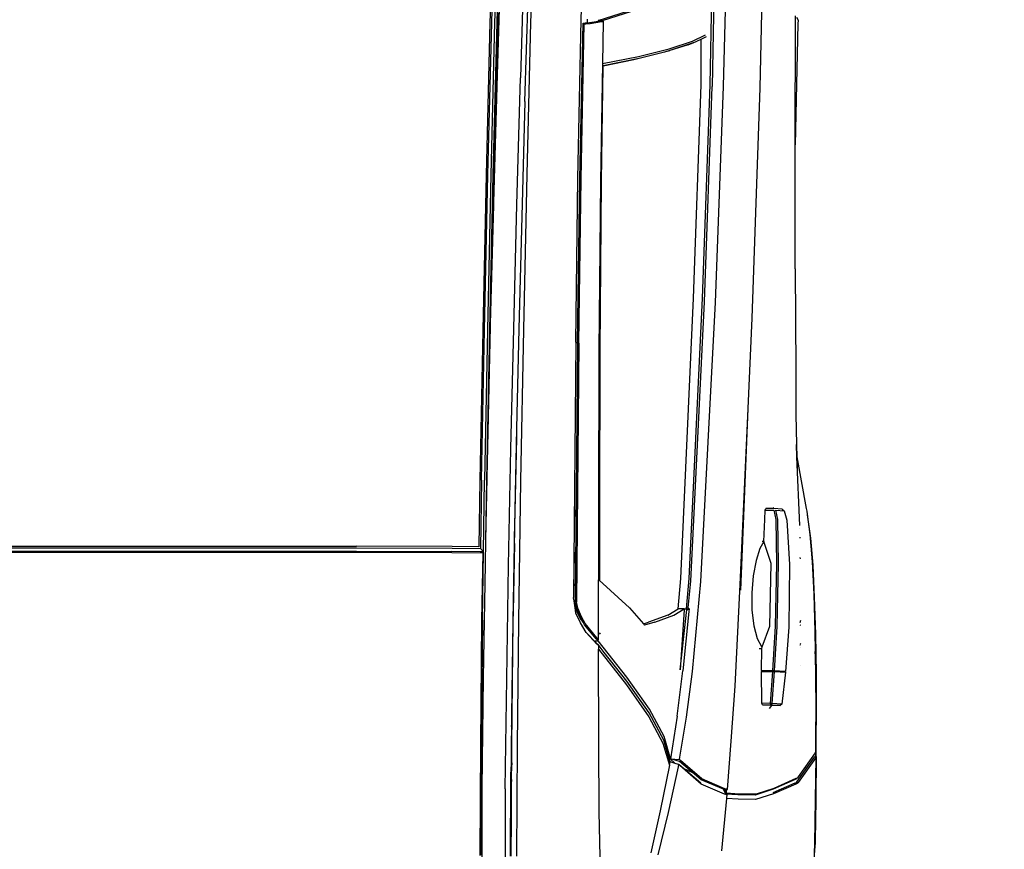
# Model space of a CAD drawing. Units: inches. Extents: x 1319 to 2030, y 219 to 1069.
# Tile 11 of 28: x 1461 to 1506, y 392 to 430. Entities that reach past the tile are written whole.
import ezdxf

# ---------------------------------------------------------------- set-up
doc = ezdxf.new("R2010")
doc.units = ezdxf.units.IN
doc.header["$MEASUREMENT"] = 0
doc.layers.get('0').update_dxf_attribs({"color": 12})
doc.layers.add('A-ANNO-DIMS', color=2, linetype='Continuous', lineweight=18)
doc.layers.add('C-PRKG-VEHC', color=8, linetype='Continuous', lineweight=13)
doc.layers.add('Edges', color=250, linetype='Continuous')
doc.styles.get("Standard").update_dxf_attribs({"font": 'arial.ttf'})
doc.dimstyles.get("Standard").update_dxf_attribs({"dimtxt": 7, "dimasz": 0.18, "dimexe": 0.18, "dimexo": 0.0625, "dimgap": 0.09, "dimtad": 0, "dimtih": 1, "dimtoh": 1, "dimzin": 0, "dimdsep": 46, "dimlunit": 3, "dimtxsty": 'Standard', "dimcen": 0.09, "dimadec": 0, "dimazin": 0, "dimtfac": 1, "dimtofl": 0, "dimtmove": 0, "dimatfit": 3, "dimfxl": 1, "dimtolj": 1, "dimtzin": 0, "dimarcsym": 0})

# ---------------------------------------------------------------- blocks, each defined once
blk = doc.blocks.new('Nissan Qashqai pl')
at = {"layer": 'Edges'}
for p, q in [((10.4339, 12.8061), (10.4573, 12.8093)), ((10.4345, 12.8062), (10.4613, 12.8099)), ((10.4573, 12.8093), (10.4889, 12.8119)), ((10.4613, 12.8099), (10.4926, 12.8125)), ((10.4889, 12.8119), (10.526, 12.8138)), ((10.4926, 12.8125), (10.5294, 12.8143)), ((10.526, 12.8138), (10.569, 12.8151)), ((10.5294, 12.8143), (10.5719, 12.8156)), ((10.569, 12.8151), (10.5919, 12.8155)), ((10.5719, 12.8156), (10.6176, 12.8164)), ((10.5919, 12.8155), (10.6151, 12.8159)), ((10.5981, 12.8157), (10.5919, 12.8155)), ((10.6174, 12.816), (10.5981, 12.8157)), ((10.6151, 12.8159), (10.6644, 12.8162)), ((10.6176, 12.8164), (10.6651, 12.8167)), ((10.6644, 12.8162), (10.7078, 12.8159)), ((10.6651, 12.8167), (10.666, 12.8167)), ((10.666, 12.8167), (10.677, 12.8167)), ((10.6729, 12.8157), (10.7082, 12.8156)), ((10.6809, 12.8167), (10.677, 12.8167)), ((10.7128, 12.8166), (10.6809, 12.8167)), ((10.7078, 12.8159), (10.7083, 12.8156)), ((10.7082, 12.8156), (10.7078, 12.8159)), ((10.7085, 12.8153), (10.7082, 12.8156)), ((10.7082, 12.8156), (10.7083, 12.8156)), ((10.7083, 12.8156), (10.7087, 12.8153)), ((10.7083, 12.8156), (10.7125, 12.8156)), ((10.7087, 12.8153), (10.7363, 12.7959)), ((10.7139, 12.8164), (10.7125, 12.8156)), ((10.7137, 12.8148), (10.7125, 12.8156)), ((10.7128, 12.8166), (10.7625, 12.8161)), ((10.7128, 12.8166), (10.724, 12.8166)), ((10.7137, 12.8148), (10.7138, 12.8147)), ((10.7418, 12.7947), (10.7138, 12.8147)), ((10.7139, 12.8164), (10.7148, 12.8157)), ((10.7628, 12.8158), (10.7139, 12.8164)), ((10.7148, 12.8157), (10.7429, 12.7956)), ((10.7685, 12.8161), (10.724, 12.8166)), ((10.7625, 12.8161), (10.7628, 12.8161)), ((10.7628, 12.8161), (10.8099, 12.8152)), ((10.8131, 12.8149), (10.7628, 12.8158)), ((10.7688, 12.8161), (10.7685, 12.8161)), ((10.8099, 12.8152), (10.7688, 12.8161)), ((10.8099, 12.8152), (10.8131, 12.8152)), ((10.8134, 12.8152), (10.8131, 12.8152)), ((10.8644, 12.8135), (10.8131, 12.8149)), ((10.8134, 12.8152), (10.8142, 12.8152)), ((10.8142, 12.8152), (10.8142, 12.8152)), ((10.8237, 12.8149), (10.8142, 12.8152)), ((10.3679, 12.7944), (10.4275, 12.8051)), ((10.4468, 12.7976), (10.3679, 12.7944)), ((10.4275, 12.8051), (10.4304, 12.8056)), ((10.4304, 12.8056), (10.4339, 12.8061)), ((10.4339, 12.8061), (10.4345, 12.8062)), ((10.4503, 12.7976), (10.4502, 12.7976)), ((10.4603, 12.7976), (10.4613, 12.7978)), ((10.4838, 12.7977), (10.4852, 12.7982)), ((10.5565, 12.7985), (10.5591, 12.7977)), ((10.5615, 12.7978), (10.5617, 12.7985)), ((10.583, 12.7984), (10.5834, 12.798)), ((10.5836, 12.798), (10.5831, 12.7984)), ((10.5847, 12.798), (10.5841, 12.7984)), ((10.5873, 12.7981), (10.5873, 12.7981)), ((10.6087, 12.7983), (10.6087, 12.7984)), ((9.8643, 12.7927), (9.8598, 12.7928)), ((9.8614, 12.7937), (9.8647, 12.7956)), ((10.0085, 12.7922), (9.8643, 12.7927)), ((9.8647, 12.7956), (9.869, 12.7954)), ((9.869, 12.7954), (10.0085, 12.7922)), ((10.0124, 12.7922), (10.0085, 12.7922)), ((10.1513, 12.7924), (10.0124, 12.7922)), ((10.1513, 12.7924), (10.2677, 12.793)), ((10.2677, 12.793), (10.3189, 12.7931)), ((10.3189, 12.7931), (10.3537, 12.7939)), ((10.3537, 12.7939), (10.3832, 12.7945)), ((10.3679, 12.7944), (10.3537, 12.7939)), ((10.4406, 12.7829), (10.4919, 12.7858)), ((10.4919, 12.7858), (10.564, 12.7851)), ((10.7363, 12.7959), (10.7376, 12.795)), ((10.7387, 12.794), (10.7376, 12.795)), ((10.7376, 12.795), (10.7378, 12.7946)), ((10.7378, 12.7946), (10.7379, 12.7945)), ((10.7378, 12.7946), (10.7385, 12.7932)), ((10.7385, 12.7932), (10.7497, 12.7679)), ((10.7387, 12.794), (10.7396, 12.7922)), ((10.7396, 12.7922), (10.7507, 12.7669)), ((10.743, 12.7939), (10.7418, 12.7947)), ((10.7432, 12.7954), (10.7426, 12.7954)), ((10.7429, 12.7956), (10.7432, 12.7954)), ((10.7434, 12.793), (10.743, 12.7939)), ((10.7441, 12.7954), (10.7432, 12.7954)), ((10.7432, 12.7954), (10.744, 12.7948)), ((10.7437, 12.7921), (10.7434, 12.793)), ((10.7438, 12.7921), (10.7437, 12.7921)), ((10.7438, 12.7921), (10.7549, 12.7666)), ((10.744, 12.7948), (10.7448, 12.793)), ((10.7448, 12.793), (10.7559, 12.7674)), ((10.4282, 12.7775), (10.4274, 12.7679)), ((10.4282, 12.7775), (10.4299, 12.7798)), ((10.4291, 12.77), (10.4299, 12.7798)), ((10.4299, 12.7798), (10.4406, 12.7829)), ((10.564, 12.7851), (10.6151, 12.7813)), ((10.615, 12.7803), (10.6142, 12.7686)), ((10.6151, 12.7813), (10.615, 12.7803)), ((10.615, 12.7676), (10.6151, 12.7803)), ((10.6151, 12.7803), (10.615, 12.7803)), ((10.6151, 12.7803), (10.6151, 12.7813)), ((10.6151, 12.7685), (10.616, 12.7812)), ((10.616, 12.7812), (10.6526, 12.7768)), ((10.6526, 12.7768), (10.6518, 12.7657)), ((10.6526, 12.7768), (10.6543, 12.7749)), ((10.6537, 12.7658), (10.6543, 12.7749)), ((10.6543, 12.7749), (10.6543, 12.7656)), ((10.4263, 12.7665), (10.4274, 12.7674)), ((10.4274, 12.7679), (10.4274, 12.7674)), ((10.4274, 12.7674), (10.4275, 12.7586)), ((10.4398, 12.7724), (10.4291, 12.77)), ((10.4291, 12.7677), (10.4398, 12.7701)), ((10.4293, 12.7579), (10.4291, 12.7677)), ((10.4909, 12.773), (10.4398, 12.7724)), ((10.4398, 12.7701), (10.4909, 12.7708)), ((10.4908, 12.7648), (10.4653, 12.7564)), ((10.563, 12.7633), (10.4908, 12.7648)), ((10.5631, 12.7715), (10.4909, 12.773)), ((10.4909, 12.7708), (10.563, 12.7692)), ((10.563, 12.7692), (10.6142, 12.7663)), ((10.5867, 12.7545), (10.563, 12.7633)), ((10.6142, 12.7686), (10.5631, 12.7715)), ((10.6142, 12.766), (10.6141, 12.7537)), ((10.6142, 12.7686), (10.6142, 12.7677)), ((10.6142, 12.7677), (10.615, 12.7676)), ((10.6142, 12.7677), (10.6142, 12.7663)), ((10.6142, 12.7663), (10.6142, 12.766)), ((10.6151, 12.7676), (10.615, 12.7676)), ((10.615, 12.7537), (10.6151, 12.7659)), ((10.6518, 12.7657), (10.6151, 12.7685)), ((10.6151, 12.7676), (10.6151, 12.7685)), ((10.6151, 12.7662), (10.6151, 12.7676)), ((10.6151, 12.7662), (10.6518, 12.7634)), ((10.6151, 12.7659), (10.6151, 12.7662)), ((10.6518, 12.7634), (10.6517, 12.754)), ((10.6536, 12.7639), (10.6518, 12.7657)), ((10.6518, 12.7657), (10.6518, 12.7634)), ((10.6518, 12.7634), (10.6536, 12.7639)), ((10.6543, 12.7656), (10.6535, 12.7546)), ((10.6535, 12.7546), (10.6536, 12.7639)), ((10.6536, 12.7639), (10.6537, 12.7658)), ((10.6537, 12.7658), (10.6543, 12.7656)), ((10.6578, 12.7628), (10.6543, 12.7656)), ((10.7497, 12.7679), (10.7565, 12.7473)), ((10.7507, 12.7669), (10.7575, 12.7462)), ((10.7559, 12.7674), (10.7626, 12.7467)), ((9.8024, 12.7549), (9.9426, 12.7518)), ((9.9426, 12.7518), (10.2081, 12.7424)), ((10.4293, 12.7579), (10.4275, 12.7586)), ((10.4398, 12.7573), (10.4293, 12.7579)), ((10.4653, 12.7564), (10.4398, 12.7573)), ((10.4653, 12.7561), (10.4652, 12.7545)), ((10.4653, 12.7564), (10.4653, 12.7561)), ((10.4653, 12.7564), (10.4653, 12.7564)), ((10.4653, 12.7564), (10.4653, 12.7561)), ((10.4653, 12.7561), (10.4653, 12.7561)), ((10.4653, 12.7561), (10.4732, 12.7517)), ((10.4732, 12.7517), (10.4871, 12.7474)), ((10.5769, 12.7484), (10.5863, 12.7537)), ((10.5863, 12.7537), (10.5867, 12.7545)), ((10.5885, 12.7538), (10.5867, 12.7545)), ((10.5885, 12.751), (10.5885, 12.7538)), ((10.6141, 12.7537), (10.5885, 12.7538)), ((10.6141, 12.7537), (10.615, 12.7537)), ((10.6517, 12.754), (10.615, 12.7537)), ((10.6535, 12.7546), (10.6517, 12.754)), ((10.2081, 12.7424), (10.312, 12.7377)), ((10.4871, 12.7474), (10.5048, 12.744)), ((10.5048, 12.744), (10.5246, 12.7423)), ((10.5246, 12.7423), (10.5445, 12.7425)), ((10.5445, 12.7425), (10.5625, 12.7446)), ((10.5625, 12.7446), (10.5769, 12.7484)), ((10.7565, 12.7473), (10.7563, 12.7273)), ((10.7575, 12.7462), (10.7572, 12.7263)), ((10.7626, 12.7467), (10.7623, 12.7269)), ((10.312, 12.7377), (10.5214, 12.7293)), ((10.312, 12.7377), (10.5147, 12.7285)), ((10.5147, 12.7285), (10.6318, 12.7228)), ((10.6318, 12.7228), (10.6955, 12.7184)), ((10.6955, 12.7184), (10.7509, 12.714)), ((10.7563, 12.7273), (10.7553, 12.7134)), ((10.7572, 12.7263), (10.7563, 12.7126)), ((10.7623, 12.7269), (10.7615, 12.7131)), ((9.9414, 12.71), (9.8143, 12.713)), ((10.19, 12.7008), (9.9414, 12.71)), ((10.7501, 12.7114), (10.7387, 12.6849)), ((10.7507, 12.7098), (10.7397, 12.684)), ((10.7563, 12.7109), (10.7449, 12.6843)), ((10.7507, 12.7132), (10.7501, 12.7114)), ((10.7506, 12.7111), (10.7507, 12.7132)), ((10.7507, 12.7132), (10.7509, 12.714)), ((10.751, 12.7132), (10.7507, 12.7132)), ((10.7511, 12.7107), (10.7507, 12.7098)), ((10.7524, 12.7106), (10.7507, 12.7098)), ((10.7522, 12.7131), (10.7509, 12.714)), ((10.7516, 12.7131), (10.7509, 12.714)), ((10.7519, 12.7128), (10.7511, 12.7107)), ((10.7522, 12.7131), (10.7516, 12.7131)), ((10.7519, 12.7128), (10.7516, 12.7131)), ((10.7526, 12.7124), (10.7519, 12.7128)), ((10.7553, 12.7134), (10.7522, 12.7131)), ((10.7524, 12.7106), (10.7526, 12.7124)), ((10.7556, 12.7122), (10.7524, 12.7106)), ((10.7526, 12.7124), (10.7526, 12.7127)), ((10.7532, 12.712), (10.7526, 12.7124)), ((10.7556, 12.7122), (10.7532, 12.712)), ((10.7561, 12.7125), (10.7556, 12.7122)), ((10.7561, 12.7125), (10.7563, 12.7126)), ((10.7563, 12.7125), (10.7561, 12.7125)), ((10.7563, 12.7123), (10.7561, 12.7123)), ((10.7563, 12.7126), (10.7573, 12.7135)), ((10.7563, 12.7126), (10.7563, 12.7125)), ((10.7569, 12.7125), (10.7563, 12.7109)), ((10.7569, 12.7125), (10.7563, 12.7125)), ((10.7563, 12.7125), (10.7563, 12.7123)), ((10.7573, 12.7135), (10.7569, 12.7125)), ((10.7573, 12.7135), (10.7604, 12.7132)), ((10.7604, 12.7132), (10.7615, 12.7131)), ((10.7615, 12.7131), (10.8218, 12.7077)), ((9.8101, 12.6993), (9.9411, 12.6966)), ((9.9393, 12.6944), (9.8119, 12.697)), ((10.1894, 12.6879), (9.9411, 12.6966)), ((10.5113, 12.6839), (10.19, 12.7008)), ((9.8891, 12.6741), (9.8818, 12.6891)), ((9.8867, 12.6842), (9.8838, 12.6901)), ((9.9393, 12.684), (9.8867, 12.6842)), ((9.8911, 12.675), (9.8867, 12.6842)), ((10.1849, 12.6857), (9.9393, 12.6944)), ((10.1849, 12.6754), (9.9393, 12.684)), ((10.5079, 12.6703), (10.1849, 12.6857)), ((10.5109, 12.6721), (10.1894, 12.6879)), ((10.6152, 12.674), (10.5113, 12.6839)), ((10.7387, 12.6849), (10.7177, 12.6604)), ((10.7449, 12.6843), (10.7232, 12.6594)), ((10.7438, 12.6836), (10.7265, 12.6635)), ((10.7397, 12.684), (10.7334, 12.6766)), ((9.8978, 12.6472), (9.8891, 12.6741)), ((9.8911, 12.6749), (9.8911, 12.675)), ((9.8931, 12.6691), (9.8911, 12.6749)), ((9.8911, 12.6749), (9.8998, 12.6481)), ((10.5079, 12.6607), (10.1849, 12.6754)), ((10.6678, 12.6672), (10.6152, 12.674)), ((10.7334, 12.6766), (10.7186, 12.6593)), ((10.7265, 12.6635), (10.7316, 12.6741)), ((9.8931, 12.669), (9.8931, 12.6691)), ((9.8931, 12.669), (9.9018, 12.6421)), ((10.543, 12.6671), (10.5079, 12.6703)), ((10.5417, 12.6693), (10.5109, 12.6721)), ((10.5417, 12.6693), (10.5427, 12.6702)), ((10.5417, 12.6693), (10.543, 12.6671)), ((10.5436, 12.6687), (10.5427, 12.6702)), ((10.5427, 12.6702), (10.5458, 12.67)), ((10.544, 12.6678), (10.543, 12.6671)), ((10.543, 12.6646), (10.543, 12.6671)), ((10.543, 12.6646), (10.543, 12.6576)), ((10.5439, 12.6646), (10.543, 12.6646)), ((10.5502, 12.6526), (10.543, 12.6646)), ((10.544, 12.6678), (10.5436, 12.6687)), ((10.5439, 12.6646), (10.613, 12.6601)), ((10.547, 12.6674), (10.544, 12.6678)), ((10.5458, 12.67), (10.6144, 12.6629)), ((10.613, 12.6601), (10.547, 12.6674)), ((10.6664, 12.6566), (10.6144, 12.6629)), ((10.7137, 12.6595), (10.6678, 12.6672)), ((10.7265, 12.6635), (10.7224, 12.6587)), ((10.543, 12.6576), (10.5079, 12.6607)), ((10.5502, 12.6456), (10.543, 12.6576)), ((10.5584, 12.6306), (10.5502, 12.6526)), ((10.6664, 12.6566), (10.7155, 12.649)), ((10.7165, 12.6591), (10.7137, 12.6595)), ((10.7186, 12.6593), (10.7155, 12.649)), ((10.7155, 12.649), (10.7165, 12.6591)), ((10.7209, 12.654), (10.7155, 12.6485)), ((10.7177, 12.6604), (10.7165, 12.6591)), ((10.7209, 12.654), (10.7192, 12.6484)), ((10.7221, 12.6581), (10.7209, 12.654)), ((10.7232, 12.6594), (10.7221, 12.6581)), ((10.7221, 12.6581), (10.7224, 12.6587)), ((10.7221, 12.6581), (10.7247, 12.6575)), ((10.7247, 12.6575), (10.7776, 12.646)), ((9.9066, 12.6119), (9.8978, 12.6472)), ((9.9086, 12.6129), (9.8998, 12.6481)), ((9.9018, 12.6421), (9.9106, 12.6068)), ((10.5502, 12.6456), (10.5584, 12.6236)), ((10.69, 12.6414), (10.6583, 12.6245)), ((10.6943, 12.641), (10.6627, 12.6241)), ((10.6671, 12.6238), (10.6976, 12.6401)), ((10.7155, 12.649), (10.69, 12.6414)), ((10.7155, 12.6473), (10.6943, 12.641)), ((10.6976, 12.6401), (10.7228, 12.6477)), ((10.7155, 12.649), (10.7155, 12.6485)), ((10.7155, 12.6485), (10.7155, 12.6473)), ((10.7192, 12.6484), (10.7155, 12.6473)), ((10.7228, 12.6477), (10.7192, 12.6484)), ((10.7228, 12.6477), (10.7754, 12.637)), ((10.7776, 12.646), (10.8264, 12.6341)), ((10.5584, 12.6306), (10.5617, 12.619)), ((10.7754, 12.637), (10.8239, 12.6261)), ((10.5419, 12.6018), (10.56, 12.6176)), ((10.56, 12.6176), (10.5584, 12.6236)), ((10.56, 12.6176), (10.5617, 12.619)), ((10.6583, 12.6245), (10.6215, 12.5986)), ((10.6627, 12.6241), (10.6261, 12.5984)), ((10.6306, 12.5982), (10.6671, 12.6238)), ((9.8652, 12.5704), (9.8516, 12.6129)), ((9.8652, 12.5654), (9.8516, 12.6079)), ((9.9149, 12.5705), (9.9066, 12.6119)), ((9.9169, 12.5714), (9.9086, 12.6129)), ((9.9106, 12.6068), (9.9177, 12.5714)), ((10.51, 12.5666), (10.5419, 12.6018)), ((10.6215, 12.5986), (10.5796, 12.5655)), ((10.5892, 12.5659), (10.6306, 12.5982)), ((10.6261, 12.5984), (10.593, 12.5726)), ((9.8652, 12.5706), (9.8664, 12.5714)), ((9.8652, 12.5706), (9.8665, 12.5695)), ((9.8652, 12.5704), (9.8652, 12.5706)), ((9.8652, 12.5704), (9.8652, 12.5704)), ((9.8652, 12.5704), (9.8652, 12.5654)), ((9.8655, 12.5687), (9.8652, 12.5704)), ((9.8665, 12.5695), (9.8664, 12.5714)), ((9.8664, 12.5714), (9.9149, 12.5705)), ((9.9149, 12.5705), (10.0505, 12.5681)), ((9.9177, 12.5714), (9.9169, 12.5714)), ((10.0501, 12.5695), (9.9177, 12.5714)), ((10.593, 12.5726), (10.584, 12.5655)), ((9.8675, 12.5555), (9.8655, 12.5687)), ((9.8686, 12.5562), (9.8665, 12.5695)), ((10.2453, 12.568), (10.0501, 12.5695)), ((10.0505, 12.5681), (10.2453, 12.5664)), ((10.4292, 12.5674), (10.2453, 12.568)), ((10.2453, 12.5664), (10.4289, 12.5658)), ((10.4289, 12.5658), (10.5092, 12.5658)), ((10.5099, 12.5674), (10.4292, 12.5674)), ((10.5099, 12.5674), (10.5092, 12.5658)), ((10.5092, 12.5658), (10.5094, 12.5658)), ((10.5094, 12.5658), (10.51, 12.5666)), ((10.5783, 12.5659), (10.5094, 12.5658)), ((10.51, 12.5666), (10.5099, 12.5674)), ((10.5764, 12.5642), (10.5598, 12.5507)), ((10.5776, 12.5633), (10.5612, 12.5498)), ((10.5834, 12.5641), (10.57, 12.5517)), ((10.57, 12.5517), (10.5821, 12.5633)), ((10.5709, 12.5675), (10.5705, 12.5671)), ((10.5719, 12.5682), (10.5709, 12.5675)), ((10.5783, 12.5659), (10.5764, 12.5642)), ((10.5776, 12.5633), (10.5783, 12.5659)), ((10.5796, 12.5655), (10.5776, 12.5633)), ((10.5796, 12.5655), (10.5783, 12.5659)), ((10.5796, 12.562), (10.5796, 12.5655)), ((10.5838, 12.5653), (10.5821, 12.5633)), ((10.584, 12.5647), (10.5834, 12.5641)), ((10.584, 12.5655), (10.5838, 12.5653)), ((10.584, 12.5655), (10.5841, 12.5655)), ((10.584, 12.5654), (10.584, 12.5655)), ((10.5847, 12.5655), (10.584, 12.5647)), ((10.584, 12.5647), (10.584, 12.5654)), ((10.5851, 12.5659), (10.5841, 12.5655)), ((10.5841, 12.5655), (10.5847, 12.5655)), ((10.5851, 12.5659), (10.5847, 12.5655)), ((10.5851, 12.5659), (10.5892, 12.5659)), ((10.6988, 12.5662), (10.5892, 12.5659)), ((10.7769, 12.5667), (10.6988, 12.5662)), ((10.858, 12.5683), (10.7769, 12.5667)), ((9.8644, 12.5459), (9.696, 12.551)), ((9.8643, 12.5532), (9.8637, 12.5532)), ((9.8677, 12.5531), (9.8643, 12.5532)), ((9.8677, 12.5531), (9.8675, 12.5555)), ((9.8678, 12.5507), (9.8677, 12.5531)), ((9.8681, 12.5482), (9.8678, 12.5507)), ((9.8681, 12.5482), (9.869, 12.5496)), ((10.0476, 12.5445), (9.8681, 12.5482)), ((9.8689, 12.5515), (9.8686, 12.5562)), ((9.869, 12.5496), (9.8689, 12.5515)), ((10.0477, 12.5459), (9.869, 12.5496)), ((10.5598, 12.5507), (10.5522, 12.5465)), ((10.5583, 12.5481), (10.5546, 12.546)), ((10.5551, 12.5457), (10.5583, 12.5481)), ((10.5612, 12.5498), (10.5583, 12.5481)), ((10.57, 12.5517), (10.5589, 12.5451)), ((10.0472, 12.5423), (9.8644, 12.5459)), ((10.2357, 12.5398), (10.0472, 12.5423)), ((10.2367, 12.5419), (10.0476, 12.5445)), ((10.2369, 12.5433), (10.0477, 12.5459)), ((10.2357, 12.5398), (10.53, 12.5373)), ((10.2367, 12.5419), (10.5351, 12.5392)), ((10.2369, 12.5433), (10.5348, 12.5406)), ((10.4153, 12.5384), (10.4176, 12.5384)), ((10.4176, 12.5384), (10.4181, 12.5384)), ((10.4181, 12.5384), (10.4552, 12.538)), ((10.4181, 12.5384), (10.4181, 12.5384)), ((10.4778, 12.5378), (10.53, 12.5373)), ((10.5301, 12.5373), (10.53, 12.5373)), ((10.5335, 12.5378), (10.5301, 12.5373)), ((10.5419, 12.5391), (10.5335, 12.5378)), ((10.5422, 12.542), (10.5348, 12.5406)), ((10.5418, 12.5405), (10.5351, 12.5392)), ((10.5424, 12.5406), (10.5418, 12.5405)), ((10.5419, 12.5391), (10.5463, 12.541)), ((10.5479, 12.54), (10.5419, 12.5391)), ((10.5522, 12.5465), (10.5422, 12.542)), ((10.5495, 12.5438), (10.5424, 12.5406)), ((10.5463, 12.541), (10.5551, 12.5457)), ((10.5589, 12.5451), (10.5479, 12.54)), ((10.5546, 12.546), (10.5495, 12.5438)), ((9.7029, 12.4926), (9.8673, 12.4878)), ((9.9583, 12.4812), (9.651, 12.4906)), ((9.6514, 12.4849), (9.9312, 12.4761)), ((9.8673, 12.4878), (10.0423, 12.4835)), ((9.9583, 12.4812), (10.091, 12.4775)), ((10.0423, 12.4835), (10.2211, 12.4795)), ((10.0776, 12.4719), (9.9312, 12.4761)), ((10.2201, 12.4683), (10.0776, 12.4719)), ((10.091, 12.4775), (10.2202, 12.4743)), ((10.3586, 12.4651), (10.2201, 12.4683)), ((10.2202, 12.4743), (10.2203, 12.4743)), ((10.2203, 12.4743), (10.3353, 12.4717)), ((10.2211, 12.4795), (10.3955, 12.4762)), ((10.3353, 12.4717), (10.4477, 12.4694)), ((10.3353, 12.4717), (10.346, 12.4714)), ((10.346, 12.4714), (10.4477, 12.4694)), ((10.3955, 12.4762), (10.5572, 12.4737)), ((10.4477, 12.4694), (10.4538, 12.4693)), ((10.4538, 12.4693), (10.4681, 12.469)), ((10.4676, 12.4691), (10.4538, 12.4693)), ((10.5566, 12.4677), (10.4676, 12.4691)), ((10.4676, 12.4691), (10.546, 12.4677)), ((10.4681, 12.469), (10.5866, 12.467)), ((10.5572, 12.4737), (10.7004, 12.4722)), ((10.7004, 12.4722), (10.8279, 12.4715)), ((9.6472, 12.4581), (9.9278, 12.4492)), ((10.4931, 12.4624), (10.3586, 12.4651)), ((10.6237, 12.4603), (10.4931, 12.4624)), ((10.546, 12.4677), (10.546, 12.4678)), ((10.546, 12.4677), (10.5576, 12.4675)), ((10.7, 12.4662), (10.5566, 12.4677)), ((10.5576, 12.4675), (10.6649, 12.4659)), ((10.5866, 12.467), (10.6649, 12.4659)), ((10.7502, 12.4586), (10.6237, 12.4603)), ((10.6649, 12.4659), (10.6786, 12.4658)), ((10.6649, 12.4659), (10.6772, 12.4657)), ((10.6786, 12.4657), (10.6772, 12.4657)), ((10.6786, 12.4658), (10.6786, 12.4662)), ((10.6786, 12.4657), (10.6786, 12.4658)), ((10.6786, 12.4658), (10.6801, 12.4657)), ((10.6786, 12.4657), (10.6801, 12.4657)), ((10.6801, 12.4662), (10.6801, 12.4657)), ((10.6801, 12.4657), (10.6801, 12.4657)), ((10.6801, 12.4657), (10.6811, 12.4657)), ((10.6801, 12.4657), (10.6811, 12.4657)), ((10.6811, 12.4662), (10.6811, 12.4657)), ((10.6811, 12.4657), (10.6811, 12.4657)), ((10.6811, 12.4657), (10.6966, 12.4654)), ((10.6811, 12.4657), (10.6991, 12.4655)), ((10.6811, 12.4657), (10.6991, 12.4655)), ((10.6966, 12.4654), (10.7144, 12.4653)), ((10.6991, 12.4655), (10.7144, 12.4653)), ((10.7201, 12.4661), (10.7, 12.4662)), ((10.7144, 12.4653), (10.7239, 12.4653)), ((10.7201, 12.4661), (10.7306, 12.4653)), ((10.7395, 12.4659), (10.7201, 12.4661)), ((10.7239, 12.4653), (10.7248, 12.4653)), ((10.7306, 12.4653), (10.7248, 12.4653)), ((10.7311, 12.4652), (10.7306, 12.4653)), ((10.7495, 12.4652), (10.7311, 12.4652)), ((10.7311, 12.4652), (10.7502, 12.4651)), ((10.7395, 12.4659), (10.7495, 12.4652)), ((10.7923, 12.4656), (10.7395, 12.4659)), ((10.8179, 12.4648), (10.7495, 12.4652)), ((10.7502, 12.4651), (10.7504, 12.4651)), ((10.7502, 12.4586), (10.968, 12.4585)), ((10.7504, 12.4651), (10.7808, 12.4649)), ((10.7808, 12.4649), (10.8179, 12.4648)), ((10.7923, 12.4652), (10.7923, 12.4656)), ((10.7933, 12.4656), (10.7923, 12.4656)), ((10.7933, 12.4652), (10.7933, 12.4656)), ((10.804, 12.4656), (10.7933, 12.4656)), ((10.804, 12.4653), (10.804, 12.4656)), ((10.8075, 12.4655), (10.804, 12.4656)), ((10.8075, 12.4655), (10.8075, 12.4653)), ((10.811, 12.4655), (10.8075, 12.4655)), ((10.811, 12.4655), (10.811, 12.4653)), ((10.8145, 12.4655), (10.811, 12.4655)), ((10.8145, 12.4653), (10.8145, 12.4655)), ((10.8279, 12.4654), (10.8145, 12.4655)), ((10.8277, 12.4647), (10.8179, 12.4648)), ((9.701, 12.4459), (9.8673, 12.441)), ((9.8673, 12.443), (9.7011, 12.4478)), ((9.7014, 12.4536), (9.8673, 12.4488)), ((9.7014, 12.4513), (9.8673, 12.4464)), ((9.9794, 12.4475), (9.8565, 12.451)), ((9.8673, 12.4488), (10.0429, 12.4444)), ((9.8673, 12.4464), (10.0429, 12.4421)), ((9.9278, 12.4492), (10.0747, 12.445)), ((10.0998, 12.4443), (9.9794, 12.4475)), ((10.043, 12.4387), (9.8673, 12.443)), ((9.8673, 12.441), (10.0431, 12.4367)), ((10.0429, 12.4444), (10.2216, 12.4404)), ((10.0429, 12.4421), (10.2215, 12.4381)), ((10.2218, 12.4347), (10.043, 12.4387)), ((10.0431, 12.4367), (10.2218, 12.4327)), ((10.0747, 12.445), (10.078, 12.4449)), ((10.078, 12.4449), (10.2146, 12.4414)), ((10.2146, 12.4414), (10.0998, 12.4443)), ((10.2146, 12.4414), (10.2175, 12.4413)), ((10.2175, 12.4413), (10.3564, 12.4382)), ((10.2215, 12.4381), (10.3945, 12.4348)), ((10.2216, 12.4404), (10.3947, 12.4371)), ((10.3947, 12.4314), (10.2218, 12.4347)), ((10.3564, 12.4382), (10.4638, 12.436)), ((10.4773, 12.4335), (10.3945, 12.4348)), ((10.3947, 12.4371), (10.4638, 12.436)), ((10.4638, 12.436), (10.4914, 12.4355)), ((10.4914, 12.4355), (10.6223, 12.4333)), ((10.2218, 12.4327), (10.3947, 12.4294)), ((10.3947, 12.4314), (10.4735, 12.4301)), ((10.3947, 12.4294), (10.4715, 12.4282)), ((10.4715, 12.4282), (10.4711, 12.3973)), ((10.4731, 12.3973), (10.4735, 12.4301)), ((10.4735, 12.4301), (10.4773, 12.4335)), ((10.4773, 12.4296), (10.4769, 12.3968)), ((10.4773, 12.4335), (10.4773, 12.4296)), ((10.4785, 12.433), (10.4773, 12.4335)), ((10.5561, 12.4323), (10.4773, 12.4335)), ((10.4781, 12.3972), (10.4785, 12.433)), ((10.5563, 12.4318), (10.4785, 12.433)), ((10.5561, 12.4323), (10.6996, 12.4308)), ((10.6999, 12.4304), (10.5563, 12.4318)), ((10.6223, 12.4333), (10.7493, 12.4316)), ((10.6996, 12.4308), (10.7722, 12.4304)), ((10.827, 12.4297), (10.6999, 12.4304)), ((10.7493, 12.4316), (11.0294, 12.4315)), ((10.7722, 12.4304), (10.7722, 12.4302)), ((10.7722, 12.4304), (10.7889, 12.4303)), ((10.7889, 12.4302), (10.7889, 12.4303)), ((10.7889, 12.4303), (10.7923, 12.4303)), ((10.7923, 12.4302), (10.7923, 12.4303)), ((10.7923, 12.4303), (10.7933, 12.4303)), ((10.7933, 12.4302), (10.7933, 12.4303)), ((10.7933, 12.4303), (10.8267, 12.4301)), ((10.4711, 12.3973), (10.4706, 12.2875)), ((10.4726, 12.2875), (10.4731, 12.3973)), ((10.4764, 12.2872), (10.4769, 12.3968)), ((10.4776, 12.2874), (10.4781, 12.3972)), ((10.4706, 11.5566), (10.4706, 12.2875)), ((10.4726, 11.5567), (10.4726, 12.2875)), ((10.4764, 11.5569), (10.4764, 12.2872)), ((10.4776, 11.5567), (10.4776, 12.2874))]:
    blk.add_line(p, q, dxfattribs=at)
blk = doc.blocks.new('car')
blk.add_blockref('Nissan Qashqai pl', (-9.7433, -11.9151))
blk = doc.blocks.new('carr')
blk.add_blockref('car', (0.5124, -0.007))
blk = doc.blocks.new('*D65')
at = {"layer": 'A-ANNO-DIMS', "color": 0, "lineweight": -2, "transparency": 16777216}
for p, q in [((1648.280254, 472.227245), (1329.112754, 472.227245)), ((1329.292754, 472.047245), (1329.292754, 431.817245)), ((1329.292754, 384.407245), (1329.292754, 424.637245)), ((1648.280254, 384.227245), (1329.112754, 384.227245))]:
    blk.add_line(p, q, dxfattribs=at)
at = {"layer": 'A-ANNO-DIMS', "color": 0, "transparency": 16777216}
for points in [[(1329.262754, 472.047245), (1329.322754, 472.047245), (1329.292754, 472.227245)], [(1329.262754, 384.407245), (1329.322754, 384.407245), (1329.292754, 384.227245)]]:
    blk.add_solid(points, dxfattribs=at)
at = {"layer": 'Defpoints', "color": 0, "transparency": 16777216}
for p in [(1329.292754, 472.227245), (1648.342754, 472.227245), (1648.342754, 384.227245)]:
    blk.add_point(p, dxfattribs=at)
at = {"layer": 'A-ANNO-DIMS', "color": 0, "transparency": 16777216, "insert": (1329.292754, 428.227245), "char_height": 7, "attachment_point": 5}
blk.add_mtext('\\A1;7\'-4"', dxfattribs=at)

msp = doc.modelspace()

# ---------------------------------------------------------------- block references
at = {"layer": 'C-PRKG-VEHC', "xscale": 39.37007874015748, "yscale": 39.37007874015748, "zscale": 39.37007874015748, "rotation": 270}
msp.add_blockref('carr', (1462.179, 454.621), dxfattribs=at)

# ---------------------------------------------------------------- dimensions: what is measured, and where the dimension line sits
at = {"layer": 'A-ANNO-DIMS'}
dim = msp.add_linear_dim(base=(1329.293, 472.227), p1=(1648.343, 384.227), p2=(1648.343, 472.227), angle=90, dimstyle='Standard', override={"dimdec": 1, "dimlfac": 1, "dimrnd": 0, "dimzin": 1, "dimdsep": 46, "dimlunit": 4, "dimfrac": 2}, dxfattribs=at)
dim.commit()
dim.dimension.update_dxf_attribs({"geometry": '*D65', "text_midpoint": (1329.293, 428.227)})

doc.saveas('drawing.dxf')
